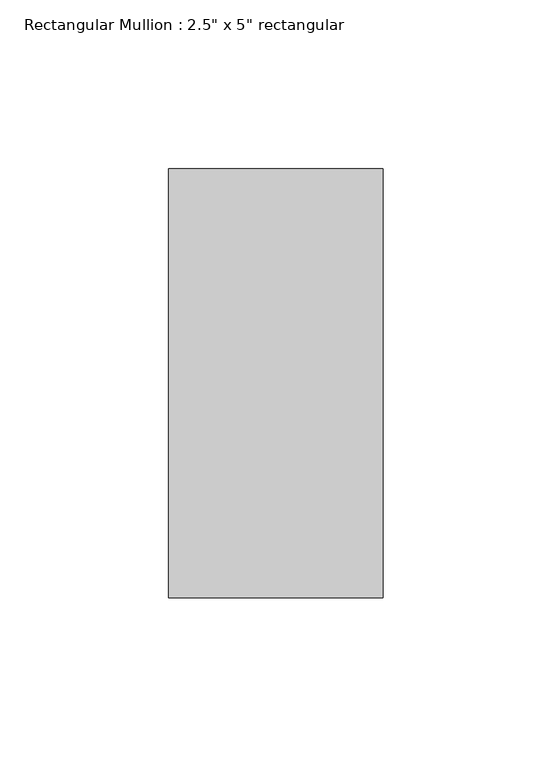
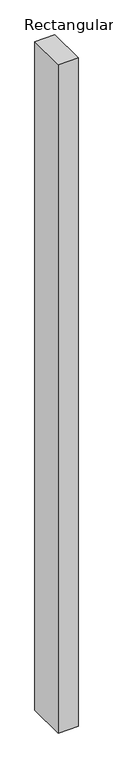
"""IFC4 building model written with IfcOpenShell, lengths in millimetres: member geometry."""

from ifc_helpers import new_model, si_unit, frame, origin, place, context, project, spatial, polyline, outline, extrude, source, transform, mapped, element, save


def member_1b8782c9(model_context):
    return source(origin(), model_context, "Body", "SweptSolid", [
        extrude(outline(polyline([(0.0, 63.5), (0.0, -63.5), (-63.5, -63.5), (-63.5, 63.5), (0.0, 63.5)])), frame((0.0, 0.0, -2241.55), z_axis=(0.0, 0.0, 1.0), x_axis=(1.0, 0.0, 0.0)), (0.0, 0.0, 1.0), 2241.55),
    ])


if __name__ == "__main__":
    model = new_model("IFC4")
    model_context = context("Model", 3, world=origin())
    ifc_project = project(units=[si_unit("LENGTHUNIT", "METRE", prefix="MILLI")], contexts=[model_context])
    site = spatial("IfcSite", under=ifc_project)
    building = spatial("IfcBuilding", under=site)
    placement = place(None, origin())
    member_shape = member_1b8782c9(model_context)
    element("IfcMember", 1, ObjectType="Rectangular Mullion : 2.5\" x 5\" rectangular", at=placement, inside=building, context=model_context, shape_type="MappedRepresentation", body=[
        mapped(member_shape, transform((0.0, 0.0, 0.0), x_axis=(1.0, 0.0, 0.0), y_axis=(0.0, 1.0, 0.0), z_axis=(0.0, 0.0, 1.0))),
    ])
    save(model, "model.ifc")

# Revit data of these elements
# Type "Rectangular Mullion : 2.5\" x 5\" rectangular"
#   built-in parameter 1007304 = 0.416667 (stored number, unit not read)
#   built-in parameter 1007301 = 0.104167 (stored number, unit not read)
#   built-in parameter 1007300 = 0.104167 (stored number, unit not read)
# Element 1 (IfcMember, "Rectangular Mullion : 2.5\" x 5\" rectangular")
#   Materials on its faces: "Aluminum"
# Materials
#   "Aluminum": class "Metal", colour RGB 247 247 247, transparency 0, Description = "Aluminum 6061", Cost = 0
